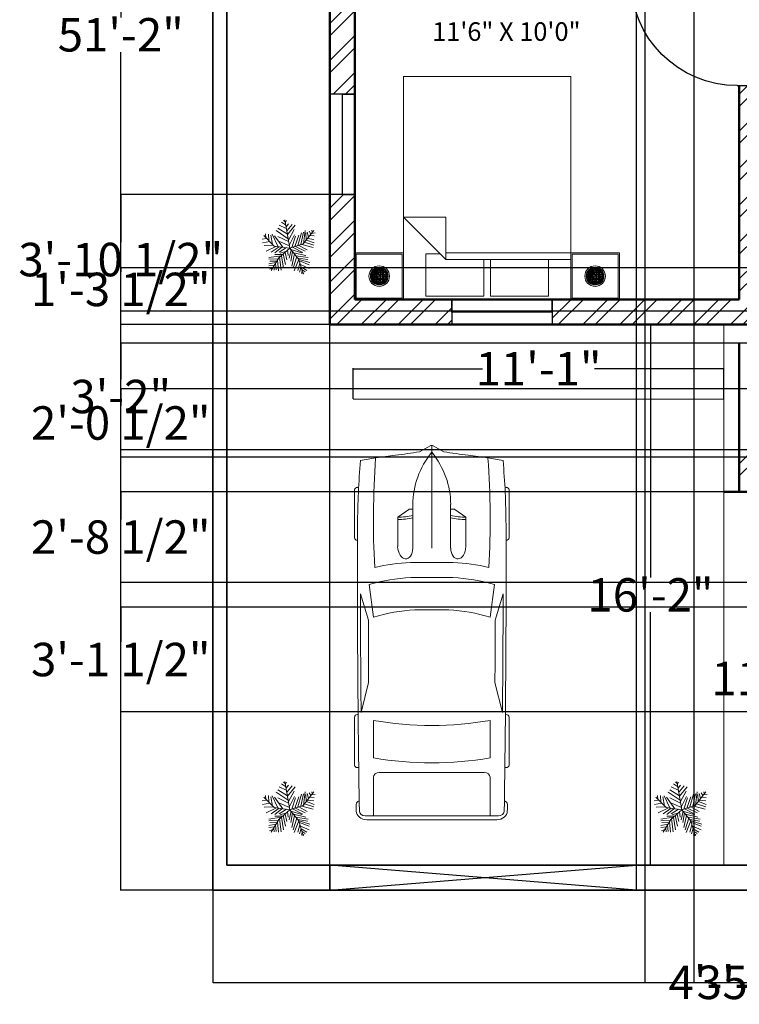
# Model space of a CAD drawing. Units: inches. Extents: x -40 to 578, y -482 to 237.
# Tile 1 of 7: x -40 to 219, y -482 to -129. Entities that reach past the tile are written whole.
import ezdxf

# ---------------------------------------------------------------- set-up
doc = ezdxf.new("R2010")
doc.units = ezdxf.units.IN
doc.header["$MEASUREMENT"] = 0
for name, color, linetype, lineweight in [('A-ANNO-DIMS', 2, 'Continuous', 18), ('A-AREA-IDEN', 240, 'Continuous', 25), ('A-FURN', 4, 'Continuous', 18), ('A-WALL-PATT', 252, 'Continuous', 13), ('C-PRKG', 8, 'Continuous', 18), ('C-PRKG-VEHI', 8, 'Continuous', 13), ('C-PROP', 3, 'Continuous', 35), ('DOORS', 2, 'Continuous', 25), ('GATE', 1, 'Continuous', 25), ('L-PLNT', 94, 'Continuous', 13), ('WALLS', 3, 'Continuous', 50), ('WINDOWS', 241, 'Continuous', 25)]:
    doc.layers.add(name, color=color, linetype=linetype, lineweight=lineweight)
doc.styles.get("Standard").update_dxf_attribs({"font": 'arial.ttf'})
doc.dimstyles.get("Standard").update_dxf_attribs({"dimtxt": 12, "dimasz": 0.18, "dimexe": 0.18, "dimexo": 0.0625, "dimgap": 0.09, "dimtad": 0, "dimtih": 1, "dimtoh": 1, "dimdec": 0, "dimzin": 0, "dimdsep": 46, "dimlunit": 3, "dimtxsty": 'Standard', "dimcen": 0.09, "dimadec": 0, "dimazin": 0, "dimtfac": 1, "dimtdec": 0, "dimtofl": 0, "dimtmove": 0, "dimatfit": 3, "dimfxl": 1, "dimtolj": 1, "dimtzin": 0, "dimarcsym": 0})

# ---------------------------------------------------------------- blocks, each defined once
blk = doc.blocks.new('Bed - Queen')
for p, q in [((0, -80.00003), (0, 0)), ((0, 0), (59.99999, 0)), ((59.99999, 0), (59.99999, -80.00003)), ((7.99999, -1.2), (28.79998, -1.2)), ((7.99999, -14.4), (7.99999, -1.2)), ((28.79998, -1.2), (28.79998, -14.4)), ((31.19999, -1.2), (51.99999, -1.2)), ((31.19999, -14.4), (31.19999, -1.2)), ((51.99999, -1.2), (51.99999, -16.4)), ((0, -14.4), (44.8, -14.4)), ((44.8, -16.8), (0, -16.8)), ((59.99999, -29.6), (44.8, -14.4)), ((44.8, -14.4), (44.8, -29.6)), ((51.99999, -16.4), (46.79936, -16.4)), ((44.8, -29.6), (59.99999, -29.6)), ((59.99999, -80.00003), (0, -80.00003))]:
    blk.add_line(p, q)
blk = doc.blocks.new('*U10')
for p, q in [((0, 0), (0, -6)), ((40, 0), (40, -6))]:
    blk.add_line(p, q)
blk.add_lwpolyline([(0, 0), (0, 40), (1.75, 40), (1.75, 0)], close=True)
blk.add_arc((0, 0), 40, 0, 90)
blk = doc.blocks.new('*U12')
for p, q in [((536, 950), (536, 936)), ((1182, 988), (568, 988)), ((1214, 950), (1214, 950)), ((2235, 810), (1899, 912)), ((3412, 904), (3030, 807)), ((3440, 942), (3440, 950)), ((3472, 988), (4087, 988)), ((4119, 950), (4119, 934)), ((1779, 801), (2195, 746)), ((4736, -851), (4736, 851)), ((4785, -832), (4785, 832)), ((3516, 746), (3994, 746)), ((4179, 670), (4179, -670)), ((4736, 746), (4242, 746)), ((820, 295), (918, 436)), ((918, 436), (1294, 436)), ((816, 241), (816, 283)), ((1496, -274), (1496, 274)), ((1690, -267), (1690, 267)), ((4736, -267), (4736, 267)), ((83, 156), (3, 10)), ((756, 241), (1313, 241)), ((2102, 216), (2102, -216)), ((0, 0), (1313, 0)), ((3, -10), (83, -156)), ((756, -241), (1313, -241)), ((816, -241), (816, -283)), ((820, -295), (918, -436)), ((918, -436), (1294, -436)), ((2195, -746), (1779, -801)), ((3994, -746), (3516, -746)), ((4242, -746), (4736, -746)), ((2235, -810), (1899, -912)), ((3412, -904), (3030, -807)), ((536, -950), (536, -936)), ((1182, -988), (568, -988)), ((1214, -950), (1214, -950)), ((3440, -942), (3440, -950)), ((3472, -988), (4087, -988)), ((4119, -950), (4119, -934))]:
    blk.add_line(p, q)
for centre, major_axis, ratio, start_param, end_param in [((6757, -699), (0, 7958), 0.842304, 1.367076, 1.39176), ((1046, -12468), (0, 13417), 0.842304, 0.00281, 0.075598), ((568, 950), (0, -37.6), 0.842304, 3.141593, 4.712389), ((1638, -268113), (0, 269063), 0.842304, -0.013397, 0.002797), ((1182, 950), (0, 37.6), 0.842304, -1.570796, 0), ((1638, -268113), (0, -269025), 0.842304, 3.133765, 3.140441), ((3472, 950), (0, -37.6), 0.842304, 3.141593, 4.712389), ((4087, 950), (0, 37.6), 0.842304, -1.570796, 0), ((4588, 910), (0, 56.4), 0.842304, -0.013017, 1.249894), ((1638, -268131), (0, 269121), 0.842304, -0.013397, -0.013017), ((4673, 851), (0, -75.2), 0.842304, 1.570796, 3.128196), ((4673, 832), (0, -133), 0.842304, 1.570796, 3.128196), ((3436, 137), (0, 2077), 0.842304, 1.245306, 1.50788), ((2433, -93125), (0, -93935), 0.842304, 3.134049, 3.144098), ((6583, -699), (0, -7755), 0.842304, 4.528606, 4.561838), ((952, -15087), (0, -15833), 0.842304, 3.096046, 3.200911), ((3414, 137), (0, -2280), 0.842304, 4.449482, 4.652344), ((3800, 71), (0, -2021), 0.842304, 4.372215, 4.640744), ((434, 0), (0, 3734), 0.842304, 4.511394, 4.913384), ((912, 0), (0, 3734), 0.842304, 4.511394, 4.913384), ((4242, 670), (0, 75.2), 0.842304, 0, 1.570796), ((-5194, 1331), (0, -6374), 0.842304, 1.385369, 1.434372), ((331, 432), (0, 696), 0.842304, 4.435146, 4.718221), ((361, 432), (0, 696), 0.842304, 4.435146, 4.718221), ((1290, 339), (161, -9), 0.603834, -1.395552, 1.581315), ((832, 283), (0, 18.8), 0.842304, 0.879714, 1.570796), ((756, -1185), (0, 1427), 0.842304, 0, 0.590319), ((16, 0), (0, -18.8), 0.842304, 4.131459, 5.293319), ((756, 1185), (0, 1427), 0.842304, 2.551274, 3.141593), ((-5194, -1331), (0, 6374), 0.842304, -1.434372, -1.385369), ((331, -432), (0, -696), 0.842304, 1.564964, 1.848039), ((361, -432), (0, -696), 0.842304, 1.564964, 1.848039), ((3800, -71), (0, -2021), 0.842304, -1.499151, -1.230623), ((832, -283), (0, -18.8), 0.842304, 4.712389, 5.403472), ((3414, -137), (0, -2280), 0.842304, -1.510751, -1.307889), ((3436, -137), (0, -2077), 0.842304, -1.50788, -1.245306), ((6583, 699), (0, 7755), 0.842304, 1.721348, 1.754579), ((6757, 699), (0, 7958), 0.842304, 1.749832, 1.774517), ((952, 15087), (0, -15833), 0.842304, -0.059319, 0.045547), ((4242, -670), (0, -75.2), 0.842304, 4.712389, 6.283185), ((2433, 93125), (0, -93935), 0.842304, -0.002505, 0.007544), ((4673, -851), (0, 75.2), 0.842304, 3.15499, 4.712389), ((4673, -832), (0, -133), 0.842304, 0.013397, 1.570796), ((1046, 12468), (0, -13417), 0.842304, -0.075598, -0.00281), ((568, -950), (0, 37.6), 0.842304, 1.570796, 3.141593), ((1638, 268113), (0, 269063), 0.842304, 3.138796, 3.15499), ((1182, -950), (0, -37.6), 0.842304, 0, 1.570796), ((1638, 268113), (0, -269025), 0.842304, 0.001152, 0.007828), ((3472, -950), (0, -37.6), 0.842304, -1.570796, 0), ((4087, -950), (0, 37.6), 0.842304, 3.141593, 4.712389), ((4588, -910), (0, -56.4), 0.842304, -1.249894, 0.013017), ((1638, 268131), (0, 269121), 0.842304, 3.15461, 3.15499)]:
    blk.add_ellipse(centre, major_axis=major_axis, ratio=ratio, start_param=start_param, end_param=end_param)
at = {"extrusion": (0, 0, -1)}
blk.add_ellipse((1290, -339), major_axis=(161, 9), ratio=0.603834, start_param=-1.395552, end_param=1.581315, dxfattribs=at)
blk = doc.blocks.new('*U14')
for p, q in [((-129.8956, 713.6638), (-626.7704, 1032.1544)), ((-185.1152, 1008.5578), (-553.1612, 1185.4942)), ((-221.9198, 1197.3052), (-433.5526, 1338.8594)), ((-258.7244, 1362.456), (-332.3336, 1421.4348)), ((0, 0), (-266.7, 1447.8)), ((-231.1146, 1315.2628), (-166.7002, 1421.4348)), ((-194.31, 1102.9442), (-65.4812, 1256.284)), ((-148.3106, 914.1968), (118.5418, 1220.9018)), ((-129.8956, 701.8528), (265.7602, 1185.4942)), ((-800.1, 114.3), (-1333.5, 647.7)), ((-1234.059, 536.7274), (-1252.4486, 737.2604)), ((-1105.2302, 725.4494), (-1077.6458, 395.1732)), ((-976.4268, 666.4706), (-884.4026, 194.6402)), ((-902.8176, 713.6638), (-617.5756, 100.2538)), ((-369.1382, 53.086), (-783.1836, 642.874)), ((-93.091, 489.5342), (-700.3796, 902.3858)), ((-617.5756, 607.4918), (-74.7014, 347.98)), ((-74.7014, 418.7444), (219.7608, 961.39)), ((-28.6766, 171.0436), (228.9556, 678.2816)), ((100.1268, 41.275), (284.1498, 619.2774)), ((256.5654, 88.4682), (449.7832, 666.4706)), ((412.9786, 147.447), (587.8068, 796.2392)), ((560.197, 182.8292), (698.2206, 819.8358)), ((685.8, 228.6), (1219.2, 914.4)), ((689.0258, 230.0224), (790.2448, 914.1968)), ((808.6344, 784.4282), (827.0494, 418.7444)), ((891.4384, 831.6214), (946.658, 572.1096)), ((983.4626, 867.0036), (1066.2666, 725.4494)), ((1029.462, 654.685), (1241.0948, 631.0884)), ((1112.2914, 760.8316), (1296.3144, 784.4282)), ((1121.4862, 925.9824), (1149.0706, 831.6214)), ((-1206.4492, 501.3198), (-1418.082, 465.9376)), ((-1031.621, 347.98), (-1399.667, 277.1902)), ((-847.598, 159.2326), (-1326.0578, 135.636)), ((-718.7946, 88.4682), (-1215.644, -147.447)), ((-543.9664, 76.6572), (-967.2066, -206.4512)), ((0, 0), (-800.1, 114.3)), ((-405.9428, 53.086), (-764.794, -241.8334)), ((0, 0), (-571.5, -495.3)), ((-166.7002, 29.4894), (-543.9664, -206.4512)), ((-525.5514, 347.98), (-28.6766, 123.8504)), ((0, 0), (685.8, 228.6)), ((0, 0), (457.2, -571.5)), ((164.5412, 41.275), (661.416, -218.2368)), ((284.1498, 88.4682), (781.0246, -147.447)), ((458.978, 147.447), (891.4384, -88.4682)), ((615.4166, 194.6402), (1185.8752, 41.275)), ((753.4148, 312.5978), (1222.6798, 159.2326)), ((845.439, 418.7444), (1241.0948, 277.1902)), ((919.0482, 501.3198), (1222.6798, 454.152)), ((-442.7474, -383.3876), (-1086.8406, -477.7486)), ((-571.5, -495.3), (-952.5, -1143)), ((-387.5278, -324.4088), (-764.794, -324.4088)), ((-525.5514, -465.963), (-451.9422, -1126.5408)), ((-166.7002, -147.447), (-507.1618, -253.619)), ((-433.5526, -383.3876), (-323.1134, -1020.3688)), ((-341.5284, -289.0012), (-221.9198, -831.6214)), ((-240.3094, -218.2368), (-157.5054, -595.7062)), ((-120.7008, -88.4682), (-93.091, -371.5766)), ((63.3222, -76.6826), (-37.8714, -513.1308)), ((44.9326, -64.897), (615.4166, -241.8334)), ((127.7366, -159.258), (54.1274, -654.685)), ((228.9556, -289.0012), (90.932, -914.1968)), ((357.759, -430.5554), (164.5412, -1020.3688)), ((192.151, -230.0224), (817.8292, -371.5766)), ((311.7596, -383.3876), (937.4378, -477.7486)), ((412.9786, -501.3452), (919.0482, -583.9206)), ((-718.7946, -737.2604), (-1086.8406, -796.2392)), ((-617.5756, -548.5384), (-1077.6458, -560.324)), ((-783.1836, -867.029), (-1077.6458, -902.4112)), ((-875.2078, -1008.5832), (-1040.8412, -1079.3476)), ((-681.9646, -666.496), (-1022.4262, -654.685)), ((-829.2084, -937.7934), (-810.7934, -1126.5408)), ((-737.1842, -784.4536), (-709.5744, -1114.7298)), ((-635.9652, -607.5172), (-580.771, -1150.1374)), ((458.978, -572.1096), (210.5406, -1161.923)), ((514.1976, -772.6426), (403.7838, -1138.3264)), ((457.2, -571.5), (685.8, -1333.5)), ((468.1982, -572.1096), (1029.462, -737.2604)), ((486.5878, -642.8994), (983.4626, -843.4324)), ((578.612, -961.39), (495.7826, -1232.7128)), ((541.8074, -831.6214), (992.6574, -1032.1544)), ((578.612, -973.1756), (873.0488, -1138.3264)), ((624.6114, -1161.923), (587.8068, -1291.6916)), ((624.6114, -1102.9442), (781.0246, -1209.1162)), ((679.8056, -1268.095), (716.6102, -1291.6916))]:
    blk.add_line(p, q)
blk = doc.blocks.new('*D15')
at = {"layer": 'A-ANNO-DIMS', "color": 0, "lineweight": -2, "transparency": 16777216}
for p, q in [((80.16, -265.23), (80.16, -254.2)), ((80.34, -254.38), (126.53, -254.38)), ((212.98, -254.38), (166.8, -254.38)), ((213.16, -265.23), (213.16, -254.2))]:
    blk.add_line(p, q, dxfattribs=at)
at = {"layer": 'A-ANNO-DIMS', "color": 0, "transparency": 16777216}
for points in [[(80.34, -254.35), (80.34, -254.41), (80.16, -254.38)], [(212.98, -254.35), (212.98, -254.41), (213.16, -254.38)]]:
    blk.add_solid(points, dxfattribs=at)
at = {"layer": 'Defpoints', "color": 0, "transparency": 16777216}
for p in [(80.16, -254.38), (80.16, -265.29), (213.16, -265.29)]:
    blk.add_point(p, dxfattribs=at)
at = {"layer": 'A-ANNO-DIMS', "color": 0, "transparency": 16777216, "insert": (146.66, -254.38), "char_height": 12, "attachment_point": 5}
blk.add_mtext('\\A1;11\'-1"', dxfattribs=at)
blk = doc.blocks.new('*D16')
at = {"layer": 'A-ANNO-DIMS', "color": 0, "lineweight": -2, "transparency": 16777216}
for p, q in [((199.73, -238.55), (186.67, -238.55)), ((186.85, -238.73), (186.85, -329.34)), ((186.85, -432.37), (186.85, -341.77)), ((199.73, -432.55), (186.67, -432.55))]:
    blk.add_line(p, q, dxfattribs=at)
at = {"layer": 'A-ANNO-DIMS', "color": 0, "transparency": 16777216}
for points in [[(186.82, -238.73), (186.88, -238.73), (186.85, -238.55)], [(186.82, -432.37), (186.88, -432.37), (186.85, -432.55)]]:
    blk.add_solid(points, dxfattribs=at)
at = {"layer": 'Defpoints', "color": 0, "transparency": 16777216}
for p in [(199.79, -238.55), (186.85, -432.55), (199.79, -432.55)]:
    blk.add_point(p, dxfattribs=at)
at = {"layer": 'A-ANNO-DIMS', "color": 0, "transparency": 16777216, "insert": (186.85, -335.55), "char_height": 12, "attachment_point": 5}
blk.add_mtext('\\A1;16\'-2"', dxfattribs=at)
blk = doc.blocks.new('*D17')
at = {"layer": 'A-ANNO-DIMS', "color": 0, "lineweight": -2, "transparency": 16777216}
for p, q in [((229.86, -298.55), (231.51, -298.55)), ((231.33, -298.73), (231.33, -359.44)), ((231.33, -432.37), (231.33, -371.67)), ((229.86, -432.55), (231.51, -432.55))]:
    blk.add_line(p, q, dxfattribs=at)
at = {"layer": 'A-ANNO-DIMS', "color": 0, "transparency": 16777216}
for points in [[(231.3, -298.73), (231.36, -298.73), (231.33, -298.55)], [(231.3, -432.37), (231.36, -432.37), (231.33, -432.55)]]:
    blk.add_solid(points, dxfattribs=at)
at = {"layer": 'Defpoints', "color": 0, "transparency": 16777216}
for p in [(229.79, -298.55), (229.79, -432.55), (231.33, -432.55)]:
    blk.add_point(p, dxfattribs=at)
at = {"layer": 'A-ANNO-DIMS', "color": 0, "transparency": 16777216, "insert": (231.33, -365.55), "char_height": 12, "attachment_point": 5}
blk.add_mtext('\\A1;11\'-2"', dxfattribs=at)
blk = doc.blocks.new('NIGHTSTAND-LAMP')
for p, q in [((6.65, 10.79), (5.56, 8.46)), ((7.17, 11.17), (5.64, 7.78)), ((7.58, 11.36), (5.82, 7.16)), ((8.24, 11.54), (6.14, 6.59)), ((6.5, 10.65), (10.99, 10.65)), ((8.75, 11.58), (6.65, 6.01)), ((6.65, 10.79), (6.65, 6.01)), ((9.21, 11.55), (7.17, 5.63)), ((7.17, 11.17), (10.32, 11.17)), ((7.17, 11.17), (7.17, 5.63)), ((9.71, 11.43), (7.58, 5.44)), ((7.58, 11.36), (7.58, 5.44)), ((8.24, 11.54), (8.24, 5.18)), ((10.22, 11.22), (8.24, 5.26)), ((8.75, 11.58), (8.75, 5.22)), ((10.75, 10.87), (8.75, 5.22)), ((9.21, 11.55), (9.21, 5.18)), ((10.99, 10.65), (9.21, 5.18)), ((9.71, 11.43), (9.71, 5.37)), ((10.22, 11.22), (10.22, 5.58)), ((10.75, 10.87), (10.75, 5.93)), ((5.56, 8.4), (11.93, 8.4)), ((5.63, 7.78), (11.87, 7.78)), ((6.14, 10.22), (5.64, 9.09)), ((5.64, 9.09), (11.85, 9.09)), ((5.64, 9.09), (5.64, 7.71)), ((5.82, 7.16), (11.68, 7.16)), ((5.83, 9.68), (11.66, 9.68)), ((6.14, 10.22), (11.36, 10.22)), ((6.14, 10.22), (6.14, 6.58)), ((11.15, 10.48), (9.71, 5.37)), ((11.36, 10.22), (10.22, 5.58)), ((11.66, 9.68), (10.75, 5.93)), ((11.15, 10.48), (11.15, 6.31)), ((11.85, 9.09), (11.15, 6.31)), ((11.81, 9.26), (11.81, 7.54)), ((6.13, 6.59), (11.37, 6.59)), ((6.6, 6.05), (10.9, 6.05)), ((7.18, 5.63), (10.31, 5.63))]:
    blk.add_line(p, q)
for points in [[(17.49, 16.8), (0, 16.8), (0, 0), (17.49, 0)], [(16.99, 16.3), (0.5, 16.3), (0.5, 0.5), (16.99, 0.5)]]:
    blk.add_lwpolyline(points, close=True)
for radius in [3.68, 3.18]:
    blk.add_circle((8.75, 8.4), radius)
blk = doc.blocks.new('WIN-36IN')
for p, q in [((9, 36), (0, 36)), ((4.5, 0), (4.5, 36)), ((4.5, 36), (9, 36)), ((9, 0), (0, 0)), ((4.5, 0), (9, 0))]:
    blk.add_line(p, q)
blk = doc.blocks.new('*D42')
at = {"layer": 'A-ANNO-DIMS', "color": 0, "lineweight": -2, "transparency": 16777216}
for p, q in [((71.78, -441.49), (71.78, 219.12)), ((181.83, -441.49), (181.83, 219.12)), ((71.96, 218.94), (110.77, 218.94)), ((181.65, 218.94), (142.84, 218.94))]:
    blk.add_line(p, q, dxfattribs=at)
at = {"layer": 'A-ANNO-DIMS', "color": 0, "transparency": 16777216}
for points in [[(71.96, 218.97), (71.96, 218.91), (71.78, 218.94)], [(181.65, 218.97), (181.65, 218.91), (181.83, 218.94)]]:
    blk.add_solid(points, dxfattribs=at)
at = {"layer": 'Defpoints', "color": 0, "transparency": 16777216}
for p in [(181.83, 218.94), (71.78, -441.55), (181.83, -441.55)]:
    blk.add_point(p, dxfattribs=at)
at = {"layer": 'A-ANNO-DIMS', "color": 0, "transparency": 16777216, "insert": (126.81, 218.94), "char_height": 12, "attachment_point": 5}
blk.add_mtext('\\A1;9\'-2"', dxfattribs=at)
blk = doc.blocks.new('*D43')
at = {"layer": 'A-ANNO-DIMS', "color": 0, "lineweight": -2, "transparency": 16777216}
for p, q in [((29.74, -441.61), (29.74, -474.78)), ((483.74, -441.61), (483.74, -474.78)), ((29.92, -474.6), (231.38, -474.6)), ((483.56, -474.6), (282.1, -474.6))]:
    blk.add_line(p, q, dxfattribs=at)
at = {"layer": 'A-ANNO-DIMS', "color": 0, "transparency": 16777216}
for points in [[(29.92, -474.57), (29.92, -474.63), (29.74, -474.6)], [(483.56, -474.57), (483.56, -474.63), (483.74, -474.6)]]:
    blk.add_solid(points, dxfattribs=at)
at = {"layer": 'Defpoints', "color": 0, "transparency": 16777216}
for p in [(29.74, -441.55), (483.74, -441.55), (483.74, -474.6)]:
    blk.add_point(p, dxfattribs=at)
at = {"layer": 'A-ANNO-DIMS', "color": 0, "transparency": 16777216, "insert": (256.74, -474.6), "char_height": 12, "attachment_point": 5}
blk.add_mtext('\\A1;37\'-10"', dxfattribs=at)
blk = doc.blocks.new('*D44')
at = {"layer": 'A-ANNO-DIMS', "color": 0, "lineweight": -2, "transparency": 16777216}
for p, q in [((29.68, 172.45), (-3.49, 172.45)), ((-3.31, 172.27), (-3.31, -128.34)), ((-3.31, -441.37), (-3.31, -140.77)), ((29.68, -441.55), (-3.49, -441.55))]:
    blk.add_line(p, q, dxfattribs=at)
at = {"layer": 'A-ANNO-DIMS', "color": 0, "transparency": 16777216}
for points in [[(-3.34, 172.27), (-3.28, 172.27), (-3.31, 172.45)], [(-3.34, -441.37), (-3.28, -441.37), (-3.31, -441.55)]]:
    blk.add_solid(points, dxfattribs=at)
at = {"layer": 'Defpoints', "color": 0, "transparency": 16777216}
for p in [(-3.31, 172.45), (29.74, 172.45), (29.74, -441.55)]:
    blk.add_point(p, dxfattribs=at)
at = {"layer": 'A-ANNO-DIMS', "color": 0, "transparency": 16777216, "insert": (-3.31, -134.55), "char_height": 12, "attachment_point": 5}
blk.add_mtext('\\A1;51\'-2"', dxfattribs=at)
blk = doc.blocks.new('*D51')
at = {"layer": 'A-ANNO-DIMS', "color": 0, "lineweight": -2, "transparency": 16777216}
for p, q in [((385.59, -298.55), (-3.49, -298.55)), ((-3.31, -298.73), (-3.31, -308.51)), ((-3.31, -330.87), (-3.31, -321.1)), ((385.59, -331.05), (-3.49, -331.05))]:
    blk.add_line(p, q, dxfattribs=at)
at = {"layer": 'A-ANNO-DIMS', "color": 0, "transparency": 16777216}
for points in [[(-3.34, -298.73), (-3.28, -298.73), (-3.31, -298.55)], [(-3.34, -330.87), (-3.28, -330.87), (-3.31, -331.05)]]:
    blk.add_solid(points, dxfattribs=at)
at = {"layer": 'Defpoints', "color": 0, "transparency": 16777216}
for p in [(385.66, -298.55), (-3.31, -331.05), (385.66, -331.05)]:
    blk.add_point(p, dxfattribs=at)
at = {"layer": 'A-ANNO-DIMS', "color": 0, "transparency": 16777216, "insert": (-3.31, -314.8), "char_height": 12, "attachment_point": 5}
blk.add_mtext('\\A1;2\'-8 1/2"', dxfattribs=at)
blk = doc.blocks.new('*D53')
at = {"layer": 'A-ANNO-DIMS', "color": 0, "lineweight": -2, "transparency": 16777216}
for p, q in [((265.59, -339.94), (-3.49, -339.94)), ((-3.31, -340.12), (-3.31, -352.45)), ((-3.31, -377.37), (-3.31, -365.04)), ((265.59, -377.55), (-3.49, -377.55))]:
    blk.add_line(p, q, dxfattribs=at)
at = {"layer": 'A-ANNO-DIMS', "color": 0, "transparency": 16777216}
for points in [[(-3.34, -340.12), (-3.28, -340.12), (-3.31, -339.94)], [(-3.34, -377.37), (-3.28, -377.37), (-3.31, -377.55)]]:
    blk.add_solid(points, dxfattribs=at)
at = {"layer": 'Defpoints', "color": 0, "transparency": 16777216}
for p in [(265.66, -339.94), (-3.31, -377.55), (265.66, -377.55)]:
    blk.add_point(p, dxfattribs=at)
at = {"layer": 'A-ANNO-DIMS', "color": 0, "transparency": 16777216, "insert": (-3.31, -358.75), "char_height": 12, "attachment_point": 5}
blk.add_mtext('\\A1;3\'-1 1/2"', dxfattribs=at)
blk = doc.blocks.new('*D54')
at = {"layer": 'A-ANNO-DIMS', "color": 0, "lineweight": -2, "transparency": 16777216}
for p, q in [((202.4, 25.39), (202.4, -474.78)), ((240.62, 25.39), (240.62, -474.78)), ((202.58, -474.6), (205.48, -474.6)), ((240.44, -474.6), (237.55, -474.6))]:
    blk.add_line(p, q, dxfattribs=at)
at = {"layer": 'A-ANNO-DIMS', "color": 0, "transparency": 16777216}
for points in [[(202.58, -474.57), (202.58, -474.63), (202.4, -474.6)], [(240.44, -474.57), (240.44, -474.63), (240.62, -474.6)]]:
    blk.add_solid(points, dxfattribs=at)
at = {"layer": 'Defpoints', "color": 0, "transparency": 16777216}
for p in [(202.4, 25.45), (240.62, 25.45), (240.62, -474.6)]:
    blk.add_point(p, dxfattribs=at)
at = {"layer": 'A-ANNO-DIMS', "color": 0, "transparency": 16777216, "insert": (221.51, -474.6), "char_height": 12, "attachment_point": 5}
blk.add_mtext('\\A1;3\'-2"', dxfattribs=at)
blk = doc.blocks.new('*D60')
at = {"layer": 'A-ANNO-DIMS', "color": 0, "lineweight": -2, "transparency": 16777216}
for p, q in [((218.68, -245.25), (-3.49, -245.25)), ((-3.31, -245.43), (-3.31, -258.14)), ((-3.31, -283.29), (-3.31, -270.58)), ((218.68, -283.47), (-3.49, -283.47))]:
    blk.add_line(p, q, dxfattribs=at)
at = {"layer": 'A-ANNO-DIMS', "color": 0, "transparency": 16777216}
for points in [[(-3.34, -245.43), (-3.28, -245.43), (-3.31, -245.25)], [(-3.34, -283.29), (-3.28, -283.29), (-3.31, -283.47)]]:
    blk.add_solid(points, dxfattribs=at)
at = {"layer": 'Defpoints', "color": 0, "transparency": 16777216}
for p in [(-3.31, -245.25), (218.74, -245.25), (218.74, -283.47)]:
    blk.add_point(p, dxfattribs=at)
at = {"layer": 'A-ANNO-DIMS', "color": 0, "transparency": 16777216, "insert": (-3.31, -264.36), "char_height": 12, "attachment_point": 5}
blk.add_mtext('\\A1;3\'-2"', dxfattribs=at)
blk = doc.blocks.new('*D70')
at = {"layer": 'A-ANNO-DIMS', "color": 0, "lineweight": -2, "transparency": 16777216}
for p, q in [((71.68, -191.89), (-3.49, -191.89)), ((-3.31, -192.07), (-3.31, -208.92)), ((-3.31, -238.37), (-3.31, -221.52)), ((71.68, -238.55), (-3.49, -238.55))]:
    blk.add_line(p, q, dxfattribs=at)
at = {"layer": 'A-ANNO-DIMS', "color": 0, "transparency": 16777216}
for points in [[(-3.34, -192.07), (-3.28, -192.07), (-3.31, -191.89)], [(-3.34, -238.37), (-3.28, -238.37), (-3.31, -238.55)]]:
    blk.add_solid(points, dxfattribs=at)
at = {"layer": 'Defpoints', "color": 0, "transparency": 16777216}
for p in [(-3.31, -191.89), (71.74, -191.89), (71.74, -238.55)]:
    blk.add_point(p, dxfattribs=at)
at = {"layer": 'A-ANNO-DIMS', "color": 0, "transparency": 16777216, "insert": (-3.31, -215.22), "char_height": 12, "attachment_point": 5}
blk.add_mtext('\\A1;3\'-10 1/2"', dxfattribs=at)
blk = doc.blocks.new('*D71')
at = {"layer": 'A-ANNO-DIMS', "color": 0, "lineweight": -2, "transparency": 16777216}
for p, q in [((184.88, -63.19), (184.88, -474.78)), ((237.97, -63.19), (237.97, -474.78)), ((185.06, -474.6), (195.15, -474.6)), ((237.79, -474.6), (227.71, -474.6))]:
    blk.add_line(p, q, dxfattribs=at)
at = {"layer": 'A-ANNO-DIMS', "color": 0, "transparency": 16777216}
for points in [[(185.06, -474.57), (185.06, -474.63), (184.88, -474.6)], [(237.79, -474.57), (237.79, -474.63), (237.97, -474.6)]]:
    blk.add_solid(points, dxfattribs=at)
at = {"layer": 'Defpoints', "color": 0, "transparency": 16777216}
for p in [(184.88, -63.12), (237.97, -63.12), (237.97, -474.6)]:
    blk.add_point(p, dxfattribs=at)
at = {"layer": 'A-ANNO-DIMS', "color": 0, "transparency": 16777216, "insert": (211.43, -474.6), "char_height": 12, "attachment_point": 5}
blk.add_mtext('\\A1;4\'-5"', dxfattribs=at)
blk = doc.blocks.new('*D74')
at = {"layer": 'A-ANNO-DIMS', "color": 0, "lineweight": -2, "transparency": 16777216}
for p, q in [((365.53, -261.64), (-3.49, -261.64)), ((-3.31, -261.82), (-3.31, -267.57)), ((-3.31, -285.9), (-3.31, -280.16)), ((371.53, -286.08), (-3.49, -286.08))]:
    blk.add_line(p, q, dxfattribs=at)
at = {"layer": 'A-ANNO-DIMS', "color": 0, "transparency": 16777216}
for points in [[(-3.34, -261.82), (-3.28, -261.82), (-3.31, -261.64)], [(-3.34, -285.9), (-3.28, -285.9), (-3.31, -286.08)]]:
    blk.add_solid(points, dxfattribs=at)
at = {"layer": 'Defpoints', "color": 0, "transparency": 16777216}
for p in [(365.59, -261.64), (-3.31, -286.08), (371.59, -286.08)]:
    blk.add_point(p, dxfattribs=at)
at = {"layer": 'A-ANNO-DIMS', "color": 0, "transparency": 16777216, "insert": (-3.31, -273.86), "char_height": 12, "attachment_point": 5}
blk.add_mtext('\\A1;2\'-0 1/2"', dxfattribs=at)
blk = doc.blocks.new('*D76')
at = {"layer": 'A-ANNO-DIMS', "color": 0, "lineweight": -2, "transparency": 16777216}
for p, q in [((310.48, -218.17), (-3.49, -218.17)), ((-3.31, -218.35), (-3.31, -219.63)), ((-3.31, -233.51), (-3.31, -232.23)), ((310.48, -233.69), (-3.49, -233.69))]:
    blk.add_line(p, q, dxfattribs=at)
at = {"layer": 'A-ANNO-DIMS', "color": 0, "transparency": 16777216}
for points in [[(-3.34, -218.35), (-3.28, -218.35), (-3.31, -218.17)], [(-3.34, -233.51), (-3.28, -233.51), (-3.31, -233.69)]]:
    blk.add_solid(points, dxfattribs=at)
at = {"layer": 'Defpoints', "color": 0, "transparency": 16777216}
for p in [(310.54, -218.17), (-3.31, -233.69), (310.54, -233.69)]:
    blk.add_point(p, dxfattribs=at)
at = {"layer": 'A-ANNO-DIMS', "color": 0, "transparency": 16777216, "insert": (-3.31, -225.93), "char_height": 12, "attachment_point": 5}
blk.add_mtext('\\A1;1\'-3 1/2"', dxfattribs=at)

msp = doc.modelspace()

# ---------------------------------------------------------------- hatches: boundary and pattern name
at = {"layer": 'A-WALL-PATT'}
h = msp.add_hatch(dxfattribs=at)
h.set_pattern_fill('ANSI32', color=256, scale=25)
h.set_pattern_definition([(45, (-1993.713, -1175.095), (-6.629126, 6.629126), []), (45, (-1989.294, -1175.095), (-6.629126, 6.629126), [])])
h.paths.add_polyline_path([(248.74, 172.45), (71.74, 172.45), (71.74, 114.63), (80.74, 114.63), (80.74, 163.45), (248.74, 163.45)])
h.paths.add_polyline_path([(253.74, 172.45), (248.74, 172.45), (248.74, 163.45), (253.74, 163.45)])
h.paths.add_polyline_path([(253.74, 163.45), (248.74, 163.45), (248.74, 25.45), (240.62, 25.45), (240.62, 20.45), (263.71, 20.45), (263.71, 25.45), (253.74, 25.45)])
h.paths.add_polyline_path([(483.74, 172.45), (253.74, 172.45), (253.74, 163.45), (426.74, 163.45), (474.74, 163.45), (474.74, 79.45), (465.23, 79.45), (465.23, 77.2), (441.23, 77.2), (441.23, 74.45), (483.74, 74.45)])
h.paths.add_polyline_path([(80.74, 78.63), (71.74, 78.63), (71.74, 3.32), (80.74, 3.32), (80.74, 20.45), (134.6, 20.45), (134.6, 25.45), (80.74, 25.45)])
h.paths.add_polyline_path([(202.4, 25.45), (158.53, 25.45), (158.53, 20.45), (202.4, 20.45)])
h.paths.add_polyline_path([(169.74, 20.45), (164.74, 20.45), (164.74, -39.55), (80.74, -39.55), (80.74, -20.68), (71.74, -20.68), (71.74, -61.38), (80.74, -61.38), (80.74, -44.55), (164.74, -44.55), (164.74, -104.55), (169.74, -104.55), (169.74, -44.55)])
h.paths.add_polyline_path([(135.96, -104.55), (80.74, -104.55), (80.74, -85.38), (71.74, -85.38), (71.74, -155.89), (80.74, -155.89), (80.74, -109.55), (135.96, -109.55)])
h.paths.add_polyline_path([(218.74, -104.55), (159.9, -104.55), (159.9, -109.55), (218.74, -109.55)])
h.paths.add_polyline_path([(223.74, -104.55), (218.74, -104.55), (218.74, -109.55), (223.74, -109.55)])
h.paths.add_polyline_path([(223.74, -109.55), (218.74, -109.55), (218.74, -114.58), (223.74, -114.58)])
h.paths.add_polyline_path([(430.74, -85.66), (421.74, -85.66), (421.74, -128.55), (223.74, -128.55), (223.74, -133.55), (421.74, -133.55), (421.74, -197.77), (430.74, -197.77)])
h.paths.add_polyline_path([(223.74, -152.8), (218.74, -152.8), (218.74, -229.55), (151.59, -229.55), (151.59, -238.55), (223.74, -238.55), (223.74, -229.55)])
h.paths.add_polyline_path([(115.59, -229.55), (98.23, -229.55), (80.74, -229.55), (80.74, -212.75), (80.74, -191.89), (71.74, -191.89), (71.74, -238.55), (115.59, -238.55)])
h.paths.add_polyline_path([(307.53, -289.55), (223.74, -289.55), (223.74, -283.47), (218.74, -283.47), (218.74, -298.55), (307.53, -298.55)])
h.paths.add_polyline_path([(421.74, -289.55), (343.53, -289.55), (343.53, -298.55), (421.74, -298.55)])
h.paths.add_polyline_path([(430.74, -367.34), (421.74, -367.34), (421.74, -377.55), (234.57, -377.55), (234.57, -386.55), (430.74, -386.55)])
h.paths.add_polyline_path([(430.74, -298.55), (430.74, -233.77), (421.74, -233.77), (421.74, -289.55), (421.74, -298.55), (421.74, -331.34), (430.74, -331.34)])
h.paths.add_polyline_path([(430.74, -11.67), (427.15, -11.67, -0.057068), (421.74, -11.05), (421.74, -49.66), (430.74, -49.66)])
h.paths.add_polyline_path([(430.74, 31.9), (421.74, 31.9), (421.74, 25.45), (301.93, 25.45), (301.93, 20.45), (421.74, 20.45), (421.74, 12.26), (430.74, 12.26)])
h.paths.add_polyline_path([(426.74, 134.23, -0.014739), (425.33, 134.19), (421.74, 134.19), (421.74, 74.45), (441.23, 74.45), (441.23, 77.2), (441.23, 79.45), (426.74, 79.45)], flags=17)
h.paths.add_polyline_path([(430.74, 74.45), (421.74, 74.45), (421.74, 67.9), (430.74, 67.9)])

# ---------------------------------------------------------------- linework, layer by layer
at = {"layer": 'C-PRKG'}
for p, q in [((213.16, -238.55), (213.16, -432.55)), ((213.16, -265.29), (80.16, -265.29))]:
    msp.add_line(p, q, dxfattribs=at)
at = {"layer": 'C-PROP'}
for p, q in [((29.74, 172.45), (29.74, -441.55)), ((34.74, 167.45), (34.74, -432.55)), ((478.74, -432.55), (34.74, -432.55)), ((483.74, -441.55), (29.74, -441.55))]:
    msp.add_line(p, q, dxfattribs=at)
at = {"layer": 'GATE'}
for p, q in [((181.83, -432.55), (71.78, -432.55)), ((71.78, -432.55), (71.78, -441.55)), ((181.83, -441.55), (71.78, -432.55)), ((71.78, -441.55), (181.83, -432.55)), ((181.83, -441.55), (181.83, -432.55)), ((71.78, -441.55), (181.83, -441.55))]:
    msp.add_line(p, q, dxfattribs=at)
at = {"layer": 'WALLS'}
for p, q in [((71.74, 172.45), (71.74, -238.55)), ((80.74, -109.55), (80.74, -229.55)), ((218.74, -152.8), (218.74, -229.55)), ((218.74, -229.55), (80.74, -229.55)), ((223.74, -238.55), (71.74, -238.55)), ((218.74, -245.25), (218.74, -298.55)), ((213.16, -289.55), (213.16, -289.55)), ((213.16, -298.55), (421.74, -298.55))]:
    msp.add_line(p, q, dxfattribs=at)

# ---------------------------------------------------------------- block references
at = {"layer": 'A-FURN', "rotation": 180}
for name, p in [('Bed - Queen', (158.23, -229.55)), ('NIGHTSTAND-LAMP', (98.23, -212.75)), ('NIGHTSTAND-LAMP', (175.72, -212.75))]:
    msp.add_blockref(name, p, dxfattribs=at)
at = {"layer": 'C-PRKG-VEHI', "xscale": 0.0280778084032927, "yscale": 0.0280778084032927, "zscale": 0.0280778084032927, "rotation": 270}
msp.add_blockref('*U12', (108.34, -281.9), dxfattribs=at)
at = {"layer": 'DOORS', "yscale": 0.9555568703817776, "zscale": 0.9555568703817776}
for p, xscale, rotation in [((218, -114.58), -0.9555568703817776, 90), ((224.47, -245.25), 0.9555568703817776, 270)]:
    msp.add_blockref('*U10', p, dxfattribs=dict(at, xscale=xscale, rotation=rotation))
at = {"layer": 'L-PLNT', "xscale": 0.0070029080995801, "yscale": 0.0070029080995801, "zscale": 0.0070029080995801}
for p in [(57.41, -211.15), (57.41, -412.68), (198.13, -412.68)]:
    msp.add_blockref('*U14', p, dxfattribs=at)
at = {"layer": 'WINDOWS'}
msp.add_blockref('WIN-36IN', (71.74, -191.89), dxfattribs=at)
at = {"layer": 'WINDOWS', "rotation": 90.0000000000001}
msp.add_blockref('WIN-36IN', (151.59, -238.55), dxfattribs=at)

# ---------------------------------------------------------------- texts
at = {"layer": 'A-AREA-IDEN'}
msp.add_text('11\'6" X 10\'0"', height=6.6698, dxfattribs=at).set_placement((108.47, -136.73))

# ---------------------------------------------------------------- dimensions: what is measured, and where the dimension line sits
at = {"layer": 'A-ANNO-DIMS'}
for base, p1, p2, override, picture, middle in [((181.8272, 218.9381), (71.7835, -441.5525), (181.8272, -441.5525), {"dimdec": 1, "dimlfac": 1, "dimrnd": 0, "dimzin": 1, "dimdsep": 46, "dimlunit": 4, "dimfrac": 2}, '*D42', (126.8054, 218.9381)), ((240.62, -474.6), (202.4, 25.45), (240.62, 25.45), {"dimdec": 1, "dimlfac": 1, "dimrnd": 0, "dimzin": 1, "dimdsep": 46, "dimlunit": 4, "dimfrac": 2}, '*D54', (221.51, -474.6)), ((237.97, -474.6), (184.88, -63.12), (237.97, -63.12), {"dimdec": 1, "dimlfac": 1, "dimrnd": 0, "dimzin": 1, "dimdsep": 46, "dimlunit": 4, "dimfrac": 2}, '*D71', (211.43, -474.6)), ((80.16, -254.38), (213.16, -265.29), (80.16, -265.29), {"dimclrd": 0, "dimclre": 0, "dimclrt": 0}, '*D15', (146.66, -254.38)), ((483.74, -474.6), (29.74, -441.55), (483.74, -441.55), {"dimdec": 1, "dimlfac": 1, "dimrnd": 0, "dimzin": 1, "dimdsep": 46, "dimlunit": 4, "dimfrac": 2}, '*D43', (256.74, -474.6))]:
    dim = msp.add_linear_dim(base=base, p1=p1, p2=p2, dimstyle='Standard', override=override, dxfattribs=at)
    dim.commit()
    dim.dimension.update_dxf_attribs({"geometry": picture, "text_midpoint": middle})
for base, p1, p2, override, picture, middle in [((-3.31, 172.45), (29.74, -441.55), (29.74, 172.45), {"dimdec": 1, "dimlfac": 1, "dimrnd": 0, "dimzin": 1, "dimdsep": 46, "dimlunit": 4, "dimfrac": 2}, '*D44', (-3.31, -134.55)), ((-3.31, -191.89), (71.74, -238.55), (71.74, -191.89), {"dimdec": 1, "dimlfac": 1, "dimrnd": 0, "dimzin": 1, "dimdsep": 46, "dimlunit": 4, "dimfrac": 2}, '*D70', (-3.31, -215.22)), ((-3.31, -233.69), (310.54, -218.17), (310.54, -233.69), {"dimdec": 1, "dimlfac": 1, "dimrnd": 0, "dimzin": 1, "dimdsep": 46, "dimlunit": 4, "dimfrac": 2}, '*D76', (-3.31, -225.93)), ((186.85, -432.55), (199.79, -238.55), (199.79, -432.55), {"dimclrd": 0, "dimclre": 0, "dimclrt": 0}, '*D16', (186.85, -335.55)), ((-3.31, -245.25), (218.74, -283.47), (218.74, -245.25), {"dimdec": 1, "dimlfac": 1, "dimrnd": 0, "dimzin": 1, "dimdsep": 46, "dimlunit": 4, "dimfrac": 2}, '*D60', (-3.31, -264.36)), ((-3.31, -286.08), (365.59, -261.64), (371.59, -286.08), {"dimdec": 1, "dimlfac": 1, "dimrnd": 0, "dimzin": 1, "dimdsep": 46, "dimlunit": 4, "dimfrac": 2}, '*D74', (-3.31, -273.86)), ((-3.31, -331.05), (385.66, -298.55), (385.66, -331.05), {"dimdec": 1, "dimlfac": 1, "dimrnd": 0, "dimzin": 1, "dimdsep": 46, "dimlunit": 4, "dimfrac": 2}, '*D51', (-3.31, -314.8)), ((231.33, -432.55), (229.79, -298.55), (229.79, -432.55), {"dimclrd": 0, "dimclre": 0, "dimclrt": 0}, '*D17', (231.33, -365.55)), ((-3.31, -377.55), (265.66, -339.94), (265.66, -377.55), {"dimdec": 1, "dimlfac": 1, "dimrnd": 0, "dimzin": 1, "dimdsep": 46, "dimlunit": 4, "dimfrac": 2}, '*D53', (-3.31, -358.75))]:
    dim = msp.add_linear_dim(base=base, p1=p1, p2=p2, angle=90, dimstyle='Standard', override=override, dxfattribs=at)
    dim.commit()
    dim.dimension.update_dxf_attribs({"geometry": picture, "text_midpoint": middle})

doc.saveas('drawing.dxf')
